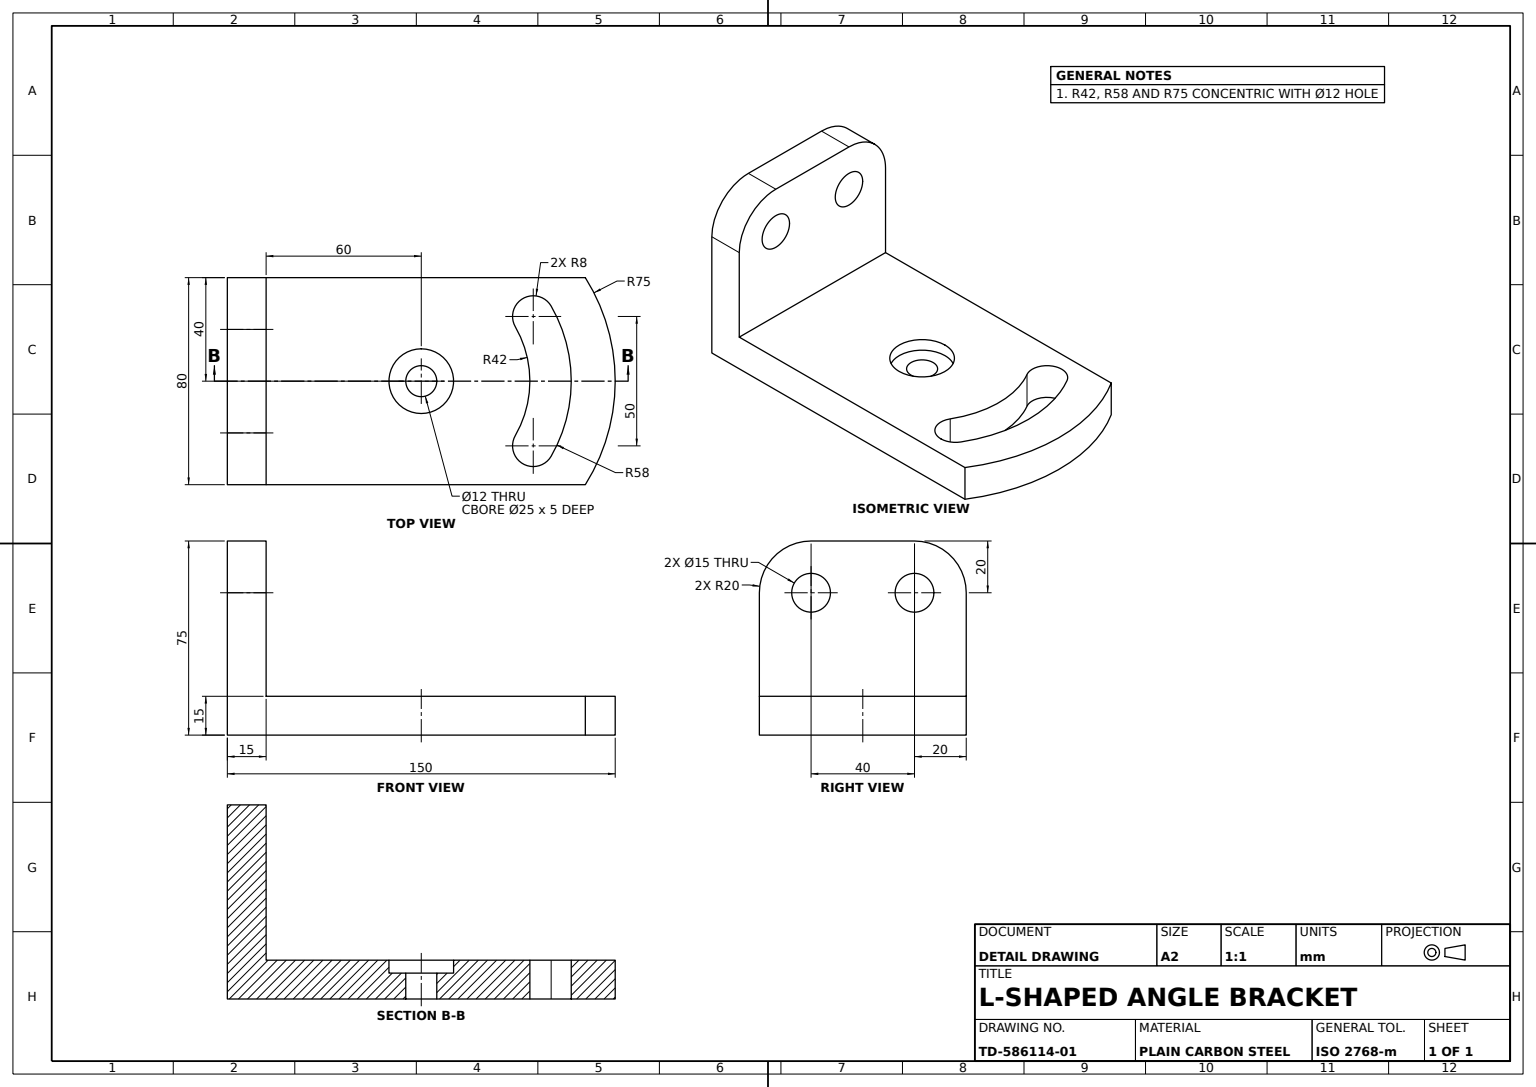
SolidWorks part; units mm, degrees
material "Plain Carbon Steel"
ref_plane "Front Plane" through (0, 0, 0) normal (0, 0, 1) x (1, 0, 0)
ref_plane "Top Plane" through (0, 0, 0) normal (0, 1, 0) x (1, 0, 0)
ref_plane "Right Plane" through (0, 0, 0) normal (1, 0, 0) x (0, 0, -1)
sketch "Base Plate Sketch" plane through (0, 0, 0) normal (0, 1, 0) x (1, 0, 0)
  line L1 (-75, 40) -> (75, 40)
  line L2 (-75, 40) -> (-75, -40)
  line L3 (-75, -40) -> (75, -40)
  line L4 (75, 40) -> (75, -40)
  line L5 (-75, 40) -> (75, -40) construction
  line L6 (-75, -40) -> (75, 40) construction
  point P0 (0, 0)
  dimension "D1" = 150
  dimension "D2" = 80
extrude "Base Plate" add sketch "Base Plate Sketch" along normal blind 15
sketch "Profile Trim Sketch" plane through (0, 15, 0) normal (0, 1, 0) x (1, 0, 0)
  line L0 (75, 40) -> (75, -40)
  line L1 (75, -40) -> (63.4429, -40)
  line L2 (-75, -40) -> (75, -40) construction
  line L3 (75, 40) -> (63.4429, 40)
  line L4 (75, 40) -> (-75, 40) construction
  circle A0 centre (0, 0) radius 75
  line M1 (75, -40) -> (75, 40)
  line M2 (75, 40) -> (-75, 40)
  line M4 (-75, -40) -> (75, -40)
  dimension "D1" = 150
extrude "Profile Trim Cut" cut sketch "Profile Trim Sketch" against normal blind 35 contours A0 L0 M2 | A0 M4 M1
sketch "Counterbore Sketch" plane through (0, 15, 0) normal (0, 1, 0) x (1, 0, 0)
  circle A0 centre (0, 0) radius 12.5
  circle A1 centre (0, 0) radius 6
  dimension "D1" = 25
  dimension "D2" = 12
extrude "Counterbore Ø25x5" cut sketch "Counterbore Sketch" against normal blind 5
sketch "Through Hole Sketch" plane through (0, 15, 0) normal (0, 1, 0) x (1, 0, 0)
  circle A1 centre (0, 0) radius 6
  circle A2 centre (0, 0) radius 6
  dimension "D1" = 0
extrude "Through Hole Cut" cut sketch "Through Hole Sketch" against normal blind 25
sketch "Arc Slot Sketch" plane through (0, 10, 0) normal (0, 1, 0) x (1, 0, 0)
  line L0 (0, 0) -> (109.1969, 0) construction
  line L1 (0, 0) -> (60.3392, 34.8369) construction
  arc A0 (43.3013, -25) -> (43.3013, 25) centre (0, 0) ccw construction
  arc A1 (50.2295, -29) -> (50.2295, 29) centre (0, 0) ccw
  arc A2 (36.3731, -21) -> (36.3731, 21) centre (0, 0) ccw
  arc A3 (36.3731, -21) -> (50.2295, -29) centre (43.3013, -25) ccw
  arc A4 (50.2295, 29) -> (36.3731, 21) centre (43.3013, 25) ccw
  point P4 (50, 0)
  dimension "D1" = 8
  dimension "D2" = 50
  dimension "D3" = 30
extrude "Arc Slot 8 R50 30deg" cut sketch "Arc Slot Sketch" against normal through all both and the other way through all contours A2 A4 A1 A3
sketch "Upright Flange Sketch" plane through (-75, 0, 0) normal (-1, 0, 0) x (0, 0, 1)
  line L2 (-40, 15) -> (-40, 55)
  line L3 (-20, 75) -> (20, 75)
  line L4 (40, 15) -> (40, 55)
  line L5 (40, 15) -> (40, 0) construction
  line L6 (-40, 15) -> (40, 15)
  arc A0 (20, 75) -> (40, 55) centre (20, 55) cw
  arc A1 (-40, 55) -> (-20, 75) centre (-20, 55) cw
  circle A2 centre (-20, 55) radius 7.5
  circle A3 centre (20, 55) radius 7.5
  dimension "D3" = 20
  dimension "D4" = 15
  dimension "D2" = 80
extrude "Upright Flange" add sketch "Upright Flange Sketch" against normal blind 15
